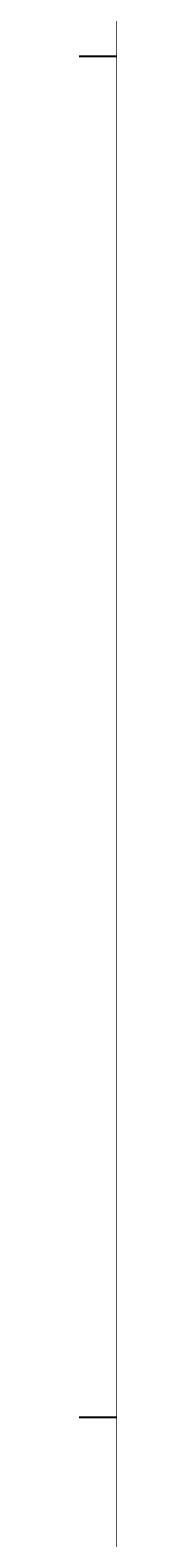
# Model space of a CAD drawing. Units: inches. Extents: x 35362 to 73946, y 43607 to 67532.
# Tile 21 of 134: x 48365 to 48371, y 46091 to 46564. Entities that reach past the tile are written whole.
import ezdxf

# ---------------------------------------------------------------- set-up
doc = ezdxf.new("R2010")
doc.units = ezdxf.units.IN
doc.header["$MEASUREMENT"] = 0
doc.layers.add('A-ANNO-DIMS', color=2, linetype='Continuous', lineweight=18)
doc.styles.get("Standard").update_dxf_attribs({"font": 'arial.ttf'})
doc.dimstyles.get("Standard").update_dxf_attribs({"dimtxt": 0.18, "dimasz": 0.18, "dimexe": 0.18, "dimexo": 0.0625, "dimgap": 0.09, "dimtad": 0, "dimtih": 1, "dimtoh": 1, "dimdec": 4, "dimzin": 0, "dimdsep": 46, "dimtxsty": 'Standard', "dimcen": 0.09, "dimadec": 0, "dimazin": 0, "dimtfac": 1, "dimtdec": 4, "dimtofl": 0, "dimtmove": 0, "dimatfit": 3, "dimfxl": 1, "dimtolj": 1, "dimtzin": 0, "dimarcsym": 0})

# ---------------------------------------------------------------- blocks, each defined once
blk = doc.blocks.new('*D5')
at = {"layer": 'A-ANNO-DIMS', "color": 0, "lineweight": -2, "transparency": 16777216}
for p, q in [((37121.95, 46919.32), (37121.95, 43606.68)), ((69871.5, 45449.83), (69871.5, 43606.68)), ((37122.13, 43606.86), (53496.29, 43606.86)), ((69871.32, 43606.86), (53497.15, 43606.86))]:
    blk.add_line(p, q, dxfattribs=at)
at = {"layer": 'A-ANNO-DIMS', "color": 0, "transparency": 16777216}
for points in [[(37122.13, 43606.89), (37122.13, 43606.83), (37121.95, 43606.86)], [(69871.32, 43606.89), (69871.32, 43606.83), (69871.5, 43606.86)]]:
    blk.add_solid(points, dxfattribs=at)
at = {"layer": 'Defpoints', "color": 0, "transparency": 16777216}
for p in [(37121.95, 46919.38), (69871.5, 45449.89), (69871.5, 43606.86)]:
    blk.add_point(p, dxfattribs=at)
at = {"layer": 'A-ANNO-DIMS', "color": 0, "transparency": 16777216, "insert": (53496.72, 43606.86), "char_height": 0.18, "attachment_point": 5}
blk.add_mtext('\\A1;32750', dxfattribs=at)
blk = doc.blocks.new('*D11')
at = {"layer": 'A-ANNO-DIMS', "color": 0, "lineweight": -2, "transparency": 16777216}
for p, q in [((47978.66, 56028.77), (47978.66, 43606.68)), ((53109.76, 56028.77), (53109.76, 43606.68)), ((47978.84, 43606.86), (50543.87, 43606.86)), ((53109.58, 43606.86), (50544.55, 43606.86))]:
    blk.add_line(p, q, dxfattribs=at)
at = {"layer": 'A-ANNO-DIMS', "color": 0, "transparency": 16777216}
for points in [[(47978.84, 43606.89), (47978.84, 43606.83), (47978.66, 43606.86)], [(53109.58, 43606.89), (53109.58, 43606.83), (53109.76, 43606.86)]]:
    blk.add_solid(points, dxfattribs=at)
at = {"layer": 'Defpoints', "color": 0, "transparency": 16777216}
for p in [(47978.66, 56028.84), (53109.76, 56028.84), (53109.76, 43606.86)]:
    blk.add_point(p, dxfattribs=at)
at = {"layer": 'A-ANNO-DIMS', "color": 0, "transparency": 16777216, "insert": (50544.21, 43606.86), "char_height": 0.18, "attachment_point": 5}
blk.add_mtext('\\A1;5131', dxfattribs=at)
blk = doc.blocks.new('*D27')
at = {"layer": 'A-ANNO-DIMS', "color": 0, "lineweight": -2, "transparency": 16777216}
for p, q in [((47978.66, 56028.77), (47978.66, 43606.68)), ((48373.49, 53428.96), (48373.49, 43606.68)), ((47978.84, 43606.86), (48175.68, 43606.86)), ((48373.31, 43606.86), (48176.47, 43606.86))]:
    blk.add_line(p, q, dxfattribs=at)
at = {"layer": 'A-ANNO-DIMS', "color": 0, "transparency": 16777216}
for points in [[(47978.84, 43606.89), (47978.84, 43606.83), (47978.66, 43606.86)], [(48373.31, 43606.89), (48373.31, 43606.83), (48373.49, 43606.86)]]:
    blk.add_solid(points, dxfattribs=at)
at = {"layer": 'Defpoints', "color": 0, "transparency": 16777216}
for p in [(47978.66, 56028.84), (48373.49, 53429.02), (48373.49, 43606.86)]:
    blk.add_point(p, dxfattribs=at)
at = {"layer": 'A-ANNO-DIMS', "color": 0, "transparency": 16777216, "insert": (48176.08, 43606.86), "char_height": 0.18, "attachment_point": 5}
blk.add_mtext('\\A1;394.8', dxfattribs=at)
blk = doc.blocks.new('*D67')
at = {"layer": 'A-ANNO-DIMS', "color": 0, "lineweight": -2, "transparency": 16777216}
for p, q in [((56873.54, 53351.53), (35361.77, 53351.53)), ((35361.95, 53351.35), (35361.95, 49400.89)), ((35361.95, 45450.07), (35361.95, 49400.53)), ((53793.58, 45449.89), (35361.77, 45449.89))]:
    blk.add_line(p, q, dxfattribs=at)
at = {"layer": 'A-ANNO-DIMS', "color": 0, "transparency": 16777216}
for points in [[(35361.92, 53351.35), (35361.98, 53351.35), (35361.95, 53351.53)], [(35361.92, 45450.07), (35361.98, 45450.07), (35361.95, 45449.89)]]:
    blk.add_solid(points, dxfattribs=at)
at = {"layer": 'Defpoints', "color": 0, "transparency": 16777216}
for p in [(35361.95, 53351.53), (56873.6, 53351.53), (53793.64, 45449.89)]:
    blk.add_point(p, dxfattribs=at)
at = {"layer": 'A-ANNO-DIMS', "color": 0, "transparency": 16777216, "insert": (35361.95, 49400.71), "char_height": 0.18, "attachment_point": 5}
blk.add_mtext('\\A1;7901.6', dxfattribs=at)
blk = doc.blocks.new('*D76')
at = {"layer": 'A-ANNO-DIMS', "color": 0, "lineweight": -2, "transparency": 16777216}
for p, q in [((54052.84, 46555.29), (35361.77, 46555.29)), ((35361.95, 46555.11), (35361.95, 46342.27)), ((35361.95, 46129.06), (35361.95, 46341.9)), ((53793.58, 46128.88), (35361.77, 46128.88))]:
    blk.add_line(p, q, dxfattribs=at)
at = {"layer": 'A-ANNO-DIMS', "color": 0, "transparency": 16777216}
for points in [[(35361.92, 46555.11), (35361.98, 46555.11), (35361.95, 46555.29)], [(35361.92, 46129.06), (35361.98, 46129.06), (35361.95, 46128.88)]]:
    blk.add_solid(points, dxfattribs=at)
at = {"layer": 'Defpoints', "color": 0, "transparency": 16777216}
for p in [(35361.95, 46555.29), (54052.9, 46555.29), (53793.64, 46128.88)]:
    blk.add_point(p, dxfattribs=at)
at = {"layer": 'A-ANNO-DIMS', "color": 0, "transparency": 16777216, "insert": (35361.95, 46342.09), "char_height": 0.18, "attachment_point": 5}
blk.add_mtext('\\A1;426.4', dxfattribs=at)
blk = doc.blocks.new('*D90')
at = {"layer": 'A-ANNO-DIMS', "color": 0, "lineweight": -2, "transparency": 16777216}
for p, q in [((53707.72, 47291.29), (35361.77, 47291.29)), ((35361.95, 47291.11), (35361.95, 46710.26)), ((35361.95, 46129.06), (35361.95, 46709.9)), ((53793.58, 46128.88), (35361.77, 46128.88))]:
    blk.add_line(p, q, dxfattribs=at)
at = {"layer": 'A-ANNO-DIMS', "color": 0, "transparency": 16777216}
for points in [[(35361.92, 47291.11), (35361.98, 47291.11), (35361.95, 47291.29)], [(35361.92, 46129.06), (35361.98, 46129.06), (35361.95, 46128.88)]]:
    blk.add_solid(points, dxfattribs=at)
at = {"layer": 'Defpoints', "color": 0, "transparency": 16777216}
for p in [(53707.78, 47291.29), (35361.95, 46128.88), (53793.64, 46128.88)]:
    blk.add_point(p, dxfattribs=at)
at = {"layer": 'A-ANNO-DIMS', "color": 0, "transparency": 16777216, "insert": (35361.95, 46710.08), "char_height": 0.18, "attachment_point": 5}
blk.add_mtext('\\A1;1162.4', dxfattribs=at)

msp = doc.modelspace()

# ---------------------------------------------------------------- dimensions: what is measured, and where the dimension line sits
at = {"layer": 'A-ANNO-DIMS'}
for base, p1, p2, override, picture, middle in [((53109.76, 43606.859), (47978.665, 56028.836), (53109.76, 56028.836), {"dimdec": 0, "dimlfac": 1, "dimrnd": 0, "dimzin": 0, "dimdsep": 46, "dimlunit": 2}, '*D11', (50544.212, 43606.859)), ((48373.492, 43606.859), (47978.665, 56028.836), (48373.492, 53429.019), {"dimdec": 1, "dimlfac": 1, "dimrnd": 0, "dimzin": 0, "dimdsep": 46, "dimlunit": 2}, '*D27', (48176.078, 43606.859)), ((69871.496, 43606.859), (37121.949, 46919.381), (69871.496, 45449.894), {"dimdec": 0, "dimlfac": 1, "dimrnd": 0, "dimzin": 0, "dimdsep": 46, "dimlunit": 2}, '*D5', (53496.723, 43606.859))]:
    dim = msp.add_linear_dim(base=base, p1=p1, p2=p2, dimstyle='Standard', override=override, dxfattribs=at)
    dim.commit()
    dim.dimension.update_dxf_attribs({"geometry": picture, "text_midpoint": middle})
for base, p1, p2, picture, middle in [((35361.949, 53351.529), (53793.638, 45449.894), (56873.602, 53351.529), '*D67', (35361.949, 49400.712)), ((35361.949, 46128.878), (53707.781, 47291.285), (53793.638, 46128.878), '*D90', (35361.949, 46710.081)), ((35361.949, 46555.293), (53793.638, 46128.878), (54052.899, 46555.293), '*D76', (35361.949, 46342.086))]:
    dim = msp.add_linear_dim(base=base, p1=p1, p2=p2, angle=90, dimstyle='Standard', override={"dimdec": 1, "dimlfac": 1, "dimrnd": 0, "dimzin": 0, "dimdsep": 46, "dimlunit": 2}, dxfattribs=at)
    dim.commit()
    dim.dimension.update_dxf_attribs({"geometry": picture, "text_midpoint": middle})

doc.saveas('drawing.dxf')
